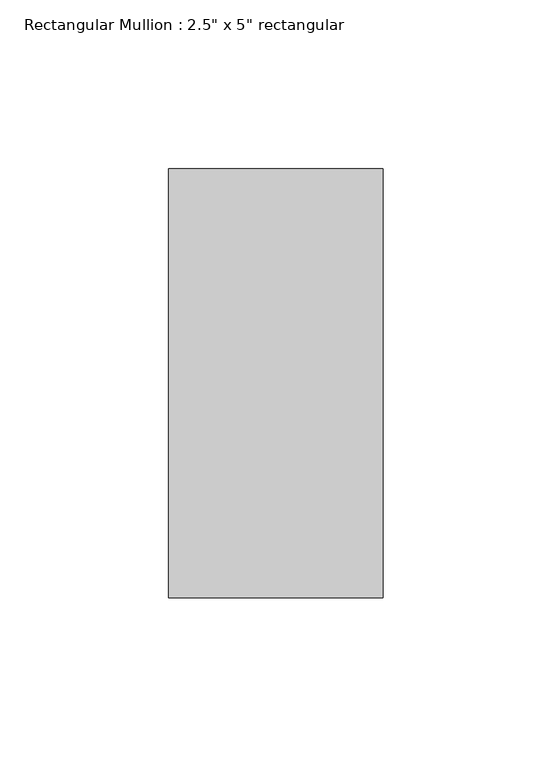
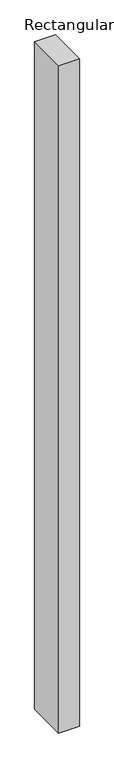
"""IFC4 building model written with IfcOpenShell, lengths in millimetres: member geometry."""

from ifc_helpers import new_model, si_unit, frame, origin, place, context, project, spatial, polyline, outline, extrude, source, transform, mapped, element, save


def member_66f4a397(model_context):
    return source(origin(), model_context, "Body", "SweptSolid", [
        extrude(outline(polyline([(31.75, 63.5), (31.75, -63.5), (-31.75, -63.5), (-31.75, 63.5), (31.75, 63.5)])), frame((0.0, 0.0, -2161.4673659), z_axis=(0.0, 0.0, 1.0), x_axis=(1.0, 0.0, 0.0)), (0.0, 0.0, 1.0), 2161.4673659),
    ])


if __name__ == "__main__":
    model = new_model("IFC4")
    model_context = context("Model", 3, world=origin())
    ifc_project = project(units=[si_unit("LENGTHUNIT", "METRE", prefix="MILLI")], contexts=[model_context])
    site = spatial("IfcSite", under=ifc_project)
    building = spatial("IfcBuilding", under=site)
    placement = place(None, origin())
    member_shape = member_66f4a397(model_context)
    element("IfcMember", 1, ObjectType="Rectangular Mullion : 2.5\" x 5\" rectangular", at=placement, inside=building, context=model_context, shape_type="MappedRepresentation", body=[
        mapped(member_shape, transform((0.0, 0.0, 0.0), x_axis=(1.0, 0.0, 0.0), y_axis=(0.0, 1.0, 0.0), z_axis=(0.0, 0.0, 1.0))),
    ])
    save(model, "model.ifc")

# Revit data of these elements
# Type "Rectangular Mullion : 2.5\" x 5\" rectangular"
#   built-in parameter 1007304 = 0.416667 (stored number, unit not read)
#   built-in parameter 1007301 = 0.104167 (stored number, unit not read)
#   built-in parameter 1007300 = 0.104167 (stored number, unit not read)
# Element 1 (IfcMember, "Rectangular Mullion : 2.5\" x 5\" rectangular")
#   Materials on its faces: "Aluminum"
# Materials
#   "Aluminum": class "Metal", colour RGB 247 247 247, transparency 0, Description = "Aluminum 6061", Cost = 0
